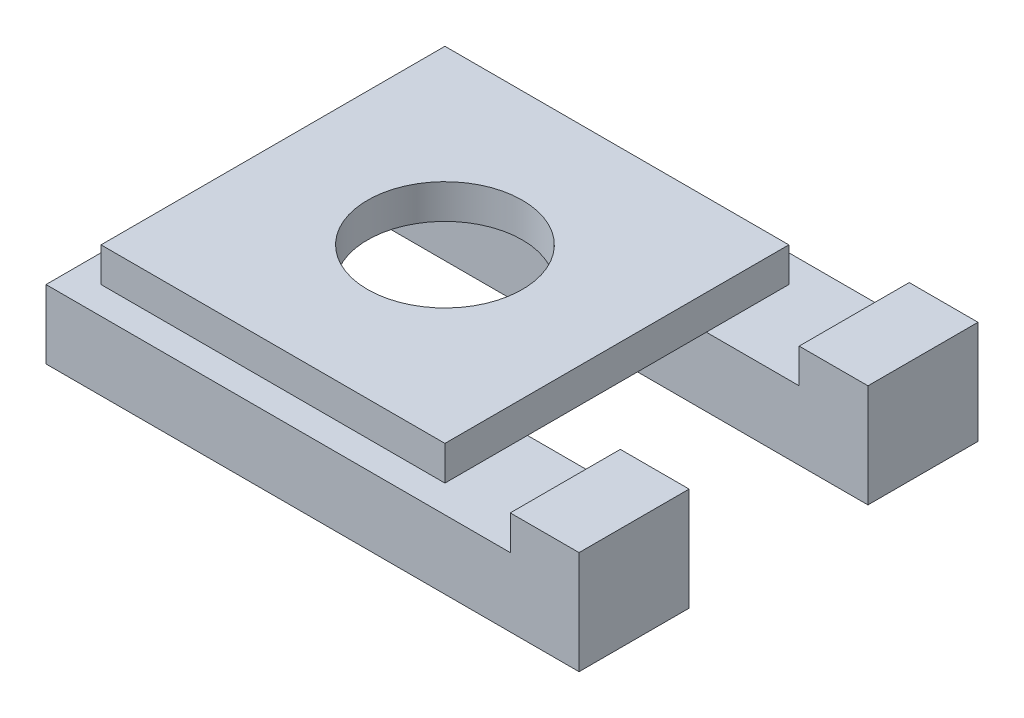
ISO-10303-21;
HEADER;
FILE_DESCRIPTION(('STEP AP214'),'2;1');
FILE_NAME('part.step','',(''),(''),'','','');
FILE_SCHEMA(('AUTOMOTIVE_DESIGN { 1 0 10303 214 1 1 1 1 }'));
ENDSEC;
DATA;
#1=APPLICATION_CONTEXT('core data for automotive mechanical design processes');
#2=APPLICATION_PROTOCOL_DEFINITION('international standard','automotive_design',2000,#1);
#3=PRODUCT_CONTEXT('',#1,'mechanical');
#4=PRODUCT('Part','Part','',(#3));
#5=PRODUCT_RELATED_PRODUCT_CATEGORY('part','',(#4));
#6=PRODUCT_DEFINITION_FORMATION('','',#4);
#7=PRODUCT_DEFINITION_CONTEXT('part definition',#1,'design');
#8=PRODUCT_DEFINITION('design','',#6,#7);
#9=PRODUCT_DEFINITION_SHAPE('','',#8);
#10=(LENGTH_UNIT() NAMED_UNIT(*) SI_UNIT(.MILLI.,.METRE.));
#11=(NAMED_UNIT(*) PLANE_ANGLE_UNIT() SI_UNIT($,.RADIAN.));
#12=(NAMED_UNIT(*) SI_UNIT($,.STERADIAN.) SOLID_ANGLE_UNIT());
#13=UNCERTAINTY_MEASURE_WITH_UNIT(LENGTH_MEASURE(1.E-05),#10,'distance_accuracy_value','');
#14=(GEOMETRIC_REPRESENTATION_CONTEXT(3) GLOBAL_UNCERTAINTY_ASSIGNED_CONTEXT((#13)) GLOBAL_UNIT_ASSIGNED_CONTEXT((#10,
#11,#12)) REPRESENTATION_CONTEXT('',''));
#15=CARTESIAN_POINT('',(0.,0.,0.));
#16=DIRECTION('',(0.,0.,1.));
#17=DIRECTION('',(1.,0.,0.));
#18=AXIS2_PLACEMENT_3D('',#15,#16,#17);
#19=CARTESIAN_POINT('',(0.,0.,0.));
#20=DIRECTION('',(0.,-1.,0.));
#21=DIRECTION('',(0.,0.,-1.));
#22=AXIS2_PLACEMENT_3D('',#19,#20,#21);
#23=PLANE('',#22);
#24=DIRECTION('',(0.,0.,1.));
#25=VECTOR('',#24,1.);
#26=CARTESIAN_POINT('',(77.,0.,-58.));
#27=LINE('',#26,#25);
#28=CARTESIAN_POINT('',(77.,0.,-58.));
#29=VERTEX_POINT('',#28);
#30=CARTESIAN_POINT('',(77.,0.,-26.));
#31=VERTEX_POINT('',#30);
#32=EDGE_CURVE('E192',#29,#31,#27,.T.);
#33=ORIENTED_EDGE('',*,*,#32,.F.);
#34=DIRECTION('',(1.,0.,0.));
#35=VECTOR('',#34,1.);
#36=CARTESIAN_POINT('',(-58.,0.,-58.));
#37=LINE('',#36,#35);
#38=CARTESIAN_POINT('',(-58.,0.,-58.));
#39=VERTEX_POINT('',#38);
#40=EDGE_CURVE('E204',#39,#29,#37,.T.);
#41=ORIENTED_EDGE('',*,*,#40,.F.);
#42=DIRECTION('',(0.,0.,-1.));
#43=VECTOR('',#42,1.);
#44=CARTESIAN_POINT('',(-58.,0.,-58.));
#45=LINE('',#44,#43);
#46=CARTESIAN_POINT('',(-58.,0.,-26.));
#47=VERTEX_POINT('',#46);
#48=EDGE_CURVE('E248',#47,#39,#45,.T.);
#49=ORIENTED_EDGE('',*,*,#48,.F.);
#50=DIRECTION('',(-1.,0.,0.));
#51=VECTOR('',#50,1.);
#52=CARTESIAN_POINT('',(-58.,0.,-26.));
#53=LINE('',#52,#51);
#54=CARTESIAN_POINT('',(-50.,0.,-26.));
#55=VERTEX_POINT('',#54);
#56=EDGE_CURVE('E255',#55,#47,#53,.T.);
#57=ORIENTED_EDGE('',*,*,#56,.F.);
#58=DIRECTION('',(0.,0.,1.));
#59=VECTOR('',#58,1.);
#60=CARTESIAN_POINT('',(-50.,0.,50.));
#61=LINE('',#60,#59);
#62=CARTESIAN_POINT('',(-50.,0.,-50.));
#63=VERTEX_POINT('',#62);
#64=EDGE_CURVE('E290',#63,#55,#61,.T.);
#65=ORIENTED_EDGE('',*,*,#64,.F.);
#66=DIRECTION('',(-1.,0.,0.));
#67=VECTOR('',#66,1.);
#68=CARTESIAN_POINT('',(-50.,0.,-50.));
#69=LINE('',#68,#67);
#70=CARTESIAN_POINT('',(50.,0.,-50.));
#71=VERTEX_POINT('',#70);
#72=EDGE_CURVE('E284',#71,#63,#69,.T.);
#73=ORIENTED_EDGE('',*,*,#72,.F.);
#74=DIRECTION('',(0.,0.,-1.));
#75=VECTOR('',#74,1.);
#76=CARTESIAN_POINT('',(50.,0.,50.));
#77=LINE('',#76,#75);
#78=CARTESIAN_POINT('',(50.,0.,-26.));
#79=VERTEX_POINT('',#78);
#80=EDGE_CURVE('E270',#79,#71,#77,.T.);
#81=ORIENTED_EDGE('',*,*,#80,.F.);
#82=EDGE_CURVE('E254',#31,#79,#53,.T.);
#83=ORIENTED_EDGE('',*,*,#82,.F.);
#84=EDGE_LOOP('',(#33,#41,#49,#57,#65,#73,#81,#83));
#85=FACE_BOUND('',#84,.T.);
#86=ADVANCED_FACE('F39',(#85),#23,.F.);
#87=CARTESIAN_POINT('',(0.,0.,0.));
#88=DIRECTION('',(0.,-1.,0.));
#89=DIRECTION('',(0.,0.,-1.));
#90=AXIS2_PLACEMENT_3D('',#87,#88,#89);
#91=PLANE('',#90);
#92=DIRECTION('',(0.,0.,1.));
#93=VECTOR('',#92,1.);
#94=CARTESIAN_POINT('',(77.,0.,26.));
#95=LINE('',#94,#93);
#96=CARTESIAN_POINT('',(77.,0.,26.));
#97=VERTEX_POINT('',#96);
#98=CARTESIAN_POINT('',(77.,0.,58.));
#99=VERTEX_POINT('',#98);
#100=EDGE_CURVE('E197',#97,#99,#95,.T.);
#101=ORIENTED_EDGE('',*,*,#100,.F.);
#102=DIRECTION('',(1.,0.,0.));
#103=VECTOR('',#102,1.);
#104=CARTESIAN_POINT('',(-58.,0.,26.));
#105=LINE('',#104,#103);
#106=CARTESIAN_POINT('',(50.,0.,26.));
#107=VERTEX_POINT('',#106);
#108=EDGE_CURVE('E51',#107,#97,#105,.T.);
#109=ORIENTED_EDGE('',*,*,#108,.F.);
#110=CARTESIAN_POINT('',(50.,0.,50.));
#111=VERTEX_POINT('',#110);
#112=EDGE_CURVE('E281',#111,#107,#77,.T.);
#113=ORIENTED_EDGE('',*,*,#112,.F.);
#114=DIRECTION('',(1.,0.,0.));
#115=VECTOR('',#114,1.);
#116=CARTESIAN_POINT('',(-50.,0.,50.));
#117=LINE('',#116,#115);
#118=CARTESIAN_POINT('',(-50.,0.,50.));
#119=VERTEX_POINT('',#118);
#120=EDGE_CURVE('E273',#119,#111,#117,.T.);
#121=ORIENTED_EDGE('',*,*,#120,.F.);
#122=CARTESIAN_POINT('',(-50.,0.,26.));
#123=VERTEX_POINT('',#122);
#124=EDGE_CURVE('E288',#123,#119,#61,.T.);
#125=ORIENTED_EDGE('',*,*,#124,.F.);
#126=CARTESIAN_POINT('',(-58.,0.,26.));
#127=VERTEX_POINT('',#126);
#128=EDGE_CURVE('E49',#127,#123,#105,.T.);
#129=ORIENTED_EDGE('',*,*,#128,.F.);
#130=DIRECTION('',(0.,0.,-1.));
#131=VECTOR('',#130,1.);
#132=CARTESIAN_POINT('',(-58.,0.,58.));
#133=LINE('',#132,#131);
#134=CARTESIAN_POINT('',(-58.,0.,58.));
#135=VERTEX_POINT('',#134);
#136=EDGE_CURVE('E177',#135,#127,#133,.T.);
#137=ORIENTED_EDGE('',*,*,#136,.F.);
#138=DIRECTION('',(-1.,0.,0.));
#139=VECTOR('',#138,1.);
#140=CARTESIAN_POINT('',(-58.,0.,58.));
#141=LINE('',#140,#139);
#142=EDGE_CURVE('E224',#99,#135,#141,.T.);
#143=ORIENTED_EDGE('',*,*,#142,.F.);
#144=EDGE_LOOP('',(#101,#109,#113,#121,#125,#129,#137,#143));
#145=FACE_BOUND('',#144,.T.);
#146=ADVANCED_FACE('F333',(#145),#91,.F.);
#147=CARTESIAN_POINT('',(0.,10.,0.));
#148=DIRECTION('',(0.,-1.,0.));
#149=DIRECTION('',(0.,0.,-1.));
#150=AXIS2_PLACEMENT_3D('',#147,#148,#149);
#151=PLANE('',#150);
#152=DIRECTION('',(0.,0.,-1.));
#153=VECTOR('',#152,1.);
#154=CARTESIAN_POINT('',(50.,10.,50.));
#155=LINE('',#154,#153);
#156=CARTESIAN_POINT('',(50.,10.,50.));
#157=VERTEX_POINT('',#156);
#158=CARTESIAN_POINT('',(50.,10.,-50.));
#159=VERTEX_POINT('',#158);
#160=EDGE_CURVE('E269',#157,#159,#155,.T.);
#161=ORIENTED_EDGE('',*,*,#160,.T.);
#162=DIRECTION('',(-1.,0.,0.));
#163=VECTOR('',#162,1.);
#164=CARTESIAN_POINT('',(-50.,10.,-50.));
#165=LINE('',#164,#163);
#166=CARTESIAN_POINT('',(-50.,10.,-50.));
#167=VERTEX_POINT('',#166);
#168=EDGE_CURVE('E272',#159,#167,#165,.T.);
#169=ORIENTED_EDGE('',*,*,#168,.T.);
#170=DIRECTION('',(0.,0.,1.));
#171=VECTOR('',#170,1.);
#172=CARTESIAN_POINT('',(-50.,10.,50.));
#173=LINE('',#172,#171);
#174=CARTESIAN_POINT('',(-50.,10.,50.));
#175=VERTEX_POINT('',#174);
#176=EDGE_CURVE('E277',#167,#175,#173,.T.);
#177=ORIENTED_EDGE('',*,*,#176,.T.);
#178=DIRECTION('',(1.,0.,0.));
#179=VECTOR('',#178,1.);
#180=CARTESIAN_POINT('',(-50.,10.,50.));
#181=LINE('',#180,#179);
#182=EDGE_CURVE('E279',#175,#157,#181,.T.);
#183=ORIENTED_EDGE('',*,*,#182,.T.);
#184=EDGE_LOOP('',(#161,#169,#177,#183));
#185=FACE_BOUND('',#184,.T.);
#186=CARTESIAN_POINT('',(0.,10.,0.));
#187=DIRECTION('',(0.,1.,0.));
#188=DIRECTION('',(0.,0.,1.));
#189=AXIS2_PLACEMENT_3D('',#186,#187,#188);
#190=CIRCLE('',#189,22.5);
#191=CARTESIAN_POINT('',(0.,10.,22.5));
#192=VERTEX_POINT('',#191);
#193=EDGE_CURVE('E262',#192,#192,#190,.T.);
#194=ORIENTED_EDGE('',*,*,#193,.F.);
#195=EDGE_LOOP('',(#194));
#196=FACE_BOUND('',#195,.T.);
#197=ADVANCED_FACE('F340',(#185,#196),#151,.F.);
#198=CARTESIAN_POINT('',(0.,0.,0.));
#199=DIRECTION('',(0.,-1.,0.));
#200=DIRECTION('',(0.,0.,-1.));
#201=AXIS2_PLACEMENT_3D('',#198,#199,#200);
#202=PLANE('',#201);
#203=EDGE_CURVE('E11',#123,#107,#105,.T.);
#204=ORIENTED_EDGE('',*,*,#203,.F.);
#205=EDGE_CURVE('E289',#55,#123,#61,.T.);
#206=ORIENTED_EDGE('',*,*,#205,.F.);
#207=EDGE_CURVE('E48',#79,#55,#53,.T.);
#208=ORIENTED_EDGE('',*,*,#207,.F.);
#209=EDGE_CURVE('E283',#107,#79,#77,.T.);
#210=ORIENTED_EDGE('',*,*,#209,.F.);
#211=EDGE_LOOP('',(#204,#206,#208,#210));
#212=FACE_BOUND('',#211,.T.);
#213=CARTESIAN_POINT('',(0.,0.,0.));
#214=DIRECTION('',(0.,1.,0.));
#215=DIRECTION('',(0.,0.,1.));
#216=AXIS2_PLACEMENT_3D('',#213,#214,#215);
#217=CIRCLE('',#216,22.5);
#218=CARTESIAN_POINT('',(0.,0.,22.5));
#219=VERTEX_POINT('',#218);
#220=EDGE_CURVE('E244',#219,#219,#217,.T.);
#221=ORIENTED_EDGE('',*,*,#220,.T.);
#222=EDGE_LOOP('',(#221));
#223=FACE_BOUND('',#222,.T.);
#224=ADVANCED_FACE('F360',(#212,#223),#202,.T.);
#225=CARTESIAN_POINT('',(50.,10.,50.));
#226=DIRECTION('',(-1.,0.,0.));
#227=DIRECTION('',(0.,0.,1.));
#228=AXIS2_PLACEMENT_3D('',#225,#226,#227);
#229=PLANE('',#228);
#230=ORIENTED_EDGE('',*,*,#112,.T.);
#231=ORIENTED_EDGE('',*,*,#209,.T.);
#232=ORIENTED_EDGE('',*,*,#80,.T.);
#233=DIRECTION('',(0.,-1.,0.));
#234=VECTOR('',#233,1.);
#235=CARTESIAN_POINT('',(50.,10.,-50.));
#236=LINE('',#235,#234);
#237=EDGE_CURVE('E43',#159,#71,#236,.T.);
#238=ORIENTED_EDGE('',*,*,#237,.F.);
#239=ORIENTED_EDGE('',*,*,#160,.F.);
#240=DIRECTION('',(0.,-1.,0.));
#241=VECTOR('',#240,1.);
#242=CARTESIAN_POINT('',(50.,10.,50.));
#243=LINE('',#242,#241);
#244=EDGE_CURVE('E278',#157,#111,#243,.T.);
#245=ORIENTED_EDGE('',*,*,#244,.T.);
#246=EDGE_LOOP('',(#230,#231,#232,#238,#239,#245));
#247=FACE_BOUND('',#246,.T.);
#248=ADVANCED_FACE('F41',(#247),#229,.F.);
#249=CARTESIAN_POINT('',(-50.,10.,-50.));
#250=DIRECTION('',(0.,0.,1.));
#251=DIRECTION('',(1.,0.,0.));
#252=AXIS2_PLACEMENT_3D('',#249,#250,#251);
#253=PLANE('',#252);
#254=ORIENTED_EDGE('',*,*,#72,.T.);
#255=DIRECTION('',(0.,-1.,0.));
#256=VECTOR('',#255,1.);
#257=CARTESIAN_POINT('',(-50.,10.,-50.));
#258=LINE('',#257,#256);
#259=EDGE_CURVE('E293',#167,#63,#258,.T.);
#260=ORIENTED_EDGE('',*,*,#259,.F.);
#261=ORIENTED_EDGE('',*,*,#168,.F.);
#262=ORIENTED_EDGE('',*,*,#237,.T.);
#263=EDGE_LOOP('',(#254,#260,#261,#262));
#264=FACE_BOUND('',#263,.T.);
#265=ADVANCED_FACE('F370',(#264),#253,.F.);
#266=CARTESIAN_POINT('',(-50.,10.,50.));
#267=DIRECTION('',(1.,0.,0.));
#268=DIRECTION('',(0.,0.,-1.));
#269=AXIS2_PLACEMENT_3D('',#266,#267,#268);
#270=PLANE('',#269);
#271=ORIENTED_EDGE('',*,*,#64,.T.);
#272=ORIENTED_EDGE('',*,*,#205,.T.);
#273=ORIENTED_EDGE('',*,*,#124,.T.);
#274=DIRECTION('',(0.,-1.,0.));
#275=VECTOR('',#274,1.);
#276=CARTESIAN_POINT('',(-50.,10.,50.));
#277=LINE('',#276,#275);
#278=EDGE_CURVE('E291',#175,#119,#277,.T.);
#279=ORIENTED_EDGE('',*,*,#278,.F.);
#280=ORIENTED_EDGE('',*,*,#176,.F.);
#281=ORIENTED_EDGE('',*,*,#259,.T.);
#282=EDGE_LOOP('',(#271,#272,#273,#279,#280,#281));
#283=FACE_BOUND('',#282,.T.);
#284=ADVANCED_FACE('F365',(#283),#270,.F.);
#285=CARTESIAN_POINT('',(-50.,10.,50.));
#286=DIRECTION('',(0.,0.,-1.));
#287=DIRECTION('',(-1.,0.,0.));
#288=AXIS2_PLACEMENT_3D('',#285,#286,#287);
#289=PLANE('',#288);
#290=ORIENTED_EDGE('',*,*,#120,.T.);
#291=ORIENTED_EDGE('',*,*,#244,.F.);
#292=ORIENTED_EDGE('',*,*,#182,.F.);
#293=ORIENTED_EDGE('',*,*,#278,.T.);
#294=EDGE_LOOP('',(#290,#291,#292,#293));
#295=FACE_BOUND('',#294,.T.);
#296=ADVANCED_FACE('F354',(#295),#289,.F.);
#297=CARTESIAN_POINT('',(0.,10.,0.));
#298=DIRECTION('',(0.,-1.,0.));
#299=DIRECTION('',(0.,0.,-1.));
#300=AXIS2_PLACEMENT_3D('',#297,#298,#299);
#301=CYLINDRICAL_SURFACE('',#300,22.5);
#302=ORIENTED_EDGE('',*,*,#193,.T.);
#303=EDGE_LOOP('',(#302));
#304=FACE_BOUND('',#303,.T.);
#305=ORIENTED_EDGE('',*,*,#220,.F.);
#306=EDGE_LOOP('',(#305));
#307=FACE_BOUND('',#306,.T.);
#308=ADVANCED_FACE('F348',(#304,#307),#301,.F.);
#309=CARTESIAN_POINT('',(-58.,-20.,-58.));
#310=DIRECTION('',(0.,0.,1.));
#311=DIRECTION('',(1.,0.,0.));
#312=AXIS2_PLACEMENT_3D('',#309,#310,#311);
#313=PLANE('',#312);
#314=ORIENTED_EDGE('',*,*,#40,.T.);
#315=DIRECTION('',(0.,-1.,0.));
#316=VECTOR('',#315,1.);
#317=CARTESIAN_POINT('',(77.,10.,-58.));
#318=LINE('',#317,#316);
#319=CARTESIAN_POINT('',(77.,10.,-58.));
#320=VERTEX_POINT('',#319);
#321=EDGE_CURVE('E187',#320,#29,#318,.T.);
#322=ORIENTED_EDGE('',*,*,#321,.F.);
#323=DIRECTION('',(-1.,0.,0.));
#324=VECTOR('',#323,1.);
#325=CARTESIAN_POINT('',(97.,10.,-58.));
#326=LINE('',#325,#324);
#327=CARTESIAN_POINT('',(97.,10.,-58.));
#328=VERTEX_POINT('',#327);
#329=EDGE_CURVE('E184',#328,#320,#326,.T.);
#330=ORIENTED_EDGE('',*,*,#329,.F.);
#331=DIRECTION('',(0.,1.,0.));
#332=VECTOR('',#331,1.);
#333=CARTESIAN_POINT('',(97.,-20.,-58.));
#334=LINE('',#333,#332);
#335=CARTESIAN_POINT('',(97.,-20.,-58.));
#336=VERTEX_POINT('',#335);
#337=EDGE_CURVE('E168',#336,#328,#334,.T.);
#338=ORIENTED_EDGE('',*,*,#337,.F.);
#339=DIRECTION('',(1.,0.,0.));
#340=VECTOR('',#339,1.);
#341=CARTESIAN_POINT('',(-58.,-20.,-58.));
#342=LINE('',#341,#340);
#343=CARTESIAN_POINT('',(-58.,-20.,-58.));
#344=VERTEX_POINT('',#343);
#345=EDGE_CURVE('E243',#344,#336,#342,.T.);
#346=ORIENTED_EDGE('',*,*,#345,.F.);
#347=DIRECTION('',(0.,1.,0.));
#348=VECTOR('',#347,1.);
#349=CARTESIAN_POINT('',(-58.,-20.,-58.));
#350=LINE('',#349,#348);
#351=EDGE_CURVE('E252',#344,#39,#350,.T.);
#352=ORIENTED_EDGE('',*,*,#351,.T.);
#353=EDGE_LOOP('',(#314,#322,#330,#338,#346,#352));
#354=FACE_BOUND('',#353,.T.);
#355=ADVANCED_FACE('F186',(#354),#313,.F.);
#356=CARTESIAN_POINT('',(97.,-20.,-58.));
#357=DIRECTION('',(-1.,0.,0.));
#358=DIRECTION('',(0.,0.,1.));
#359=AXIS2_PLACEMENT_3D('',#356,#357,#358);
#360=PLANE('',#359);
#361=ORIENTED_EDGE('',*,*,#337,.T.);
#362=DIRECTION('',(0.,0.,-1.));
#363=VECTOR('',#362,1.);
#364=CARTESIAN_POINT('',(97.,10.,-58.));
#365=LINE('',#364,#363);
#366=CARTESIAN_POINT('',(97.,10.,-26.));
#367=VERTEX_POINT('',#366);
#368=EDGE_CURVE('E175',#367,#328,#365,.T.);
#369=ORIENTED_EDGE('',*,*,#368,.F.);
#370=DIRECTION('',(0.,1.,0.));
#371=VECTOR('',#370,1.);
#372=CARTESIAN_POINT('',(97.,-20.,-26.));
#373=LINE('',#372,#371);
#374=CARTESIAN_POINT('',(97.,-20.,-26.));
#375=VERTEX_POINT('',#374);
#376=EDGE_CURVE('E182',#375,#367,#373,.T.);
#377=ORIENTED_EDGE('',*,*,#376,.F.);
#378=DIRECTION('',(0.,0.,1.));
#379=VECTOR('',#378,1.);
#380=CARTESIAN_POINT('',(97.,-20.,-58.));
#381=LINE('',#380,#379);
#382=EDGE_CURVE('E178',#336,#375,#381,.T.);
#383=ORIENTED_EDGE('',*,*,#382,.F.);
#384=EDGE_LOOP('',(#361,#369,#377,#383));
#385=FACE_BOUND('',#384,.T.);
#386=ADVANCED_FACE('F172',(#385),#360,.F.);
#387=CARTESIAN_POINT('',(-58.,-20.,-26.));
#388=DIRECTION('',(0.,0.,-1.));
#389=DIRECTION('',(-1.,0.,0.));
#390=AXIS2_PLACEMENT_3D('',#387,#388,#389);
#391=PLANE('',#390);
#392=ORIENTED_EDGE('',*,*,#376,.T.);
#393=DIRECTION('',(1.,0.,0.));
#394=VECTOR('',#393,1.);
#395=CARTESIAN_POINT('',(97.,10.,-26.));
#396=LINE('',#395,#394);
#397=CARTESIAN_POINT('',(77.,10.,-26.));
#398=VERTEX_POINT('',#397);
#399=EDGE_CURVE('E194',#398,#367,#396,.T.);
#400=ORIENTED_EDGE('',*,*,#399,.F.);
#401=DIRECTION('',(0.,-1.,0.));
#402=VECTOR('',#401,1.);
#403=CARTESIAN_POINT('',(77.,10.,-26.));
#404=LINE('',#403,#402);
#405=EDGE_CURVE('E59',#398,#31,#404,.T.);
#406=ORIENTED_EDGE('',*,*,#405,.T.);
#407=ORIENTED_EDGE('',*,*,#82,.T.);
#408=ORIENTED_EDGE('',*,*,#207,.T.);
#409=ORIENTED_EDGE('',*,*,#56,.T.);
#410=DIRECTION('',(0.,1.,0.));
#411=VECTOR('',#410,1.);
#412=CARTESIAN_POINT('',(-58.,-20.,-26.));
#413=LINE('',#412,#411);
#414=CARTESIAN_POINT('',(-58.,-20.,-26.));
#415=VERTEX_POINT('',#414);
#416=EDGE_CURVE('E257',#415,#47,#413,.T.);
#417=ORIENTED_EDGE('',*,*,#416,.F.);
#418=DIRECTION('',(-1.,0.,0.));
#419=VECTOR('',#418,1.);
#420=CARTESIAN_POINT('',(-58.,-20.,-26.));
#421=LINE('',#420,#419);
#422=EDGE_CURVE('E246',#375,#415,#421,.T.);
#423=ORIENTED_EDGE('',*,*,#422,.F.);
#424=EDGE_LOOP('',(#392,#400,#406,#407,#408,#409,#417,#423));
#425=FACE_BOUND('',#424,.T.);
#426=ADVANCED_FACE('F310',(#425),#391,.F.);
#427=CARTESIAN_POINT('',(-58.,-20.,-58.));
#428=DIRECTION('',(1.,0.,0.));
#429=DIRECTION('',(0.,0.,-1.));
#430=AXIS2_PLACEMENT_3D('',#427,#428,#429);
#431=PLANE('',#430);
#432=ORIENTED_EDGE('',*,*,#48,.T.);
#433=ORIENTED_EDGE('',*,*,#351,.F.);
#434=DIRECTION('',(0.,0.,-1.));
#435=VECTOR('',#434,1.);
#436=CARTESIAN_POINT('',(-58.,-20.,-58.));
#437=LINE('',#436,#435);
#438=EDGE_CURVE('E247',#415,#344,#437,.T.);
#439=ORIENTED_EDGE('',*,*,#438,.F.);
#440=ORIENTED_EDGE('',*,*,#416,.T.);
#441=EDGE_LOOP('',(#432,#433,#439,#440));
#442=FACE_BOUND('',#441,.T.);
#443=ADVANCED_FACE('F312',(#442),#431,.F.);
#444=CARTESIAN_POINT('',(0.,-20.,0.));
#445=DIRECTION('',(0.,-1.,0.));
#446=DIRECTION('',(0.,0.,-1.));
#447=AXIS2_PLACEMENT_3D('',#444,#445,#446);
#448=PLANE('',#447);
#449=ORIENTED_EDGE('',*,*,#345,.T.);
#450=ORIENTED_EDGE('',*,*,#382,.T.);
#451=ORIENTED_EDGE('',*,*,#422,.T.);
#452=ORIENTED_EDGE('',*,*,#438,.T.);
#453=EDGE_LOOP('',(#449,#450,#451,#452));
#454=FACE_BOUND('',#453,.T.);
#455=ADVANCED_FACE('F321',(#454),#448,.T.);
#456=CARTESIAN_POINT('',(-58.,-20.,58.));
#457=DIRECTION('',(1.,0.,0.));
#458=DIRECTION('',(0.,0.,-1.));
#459=AXIS2_PLACEMENT_3D('',#456,#457,#458);
#460=PLANE('',#459);
#461=ORIENTED_EDGE('',*,*,#136,.T.);
#462=DIRECTION('',(0.,1.,0.));
#463=VECTOR('',#462,1.);
#464=CARTESIAN_POINT('',(-58.,-20.,26.));
#465=LINE('',#464,#463);
#466=CARTESIAN_POINT('',(-58.,-20.,26.));
#467=VERTEX_POINT('',#466);
#468=EDGE_CURVE('E238',#467,#127,#465,.T.);
#469=ORIENTED_EDGE('',*,*,#468,.F.);
#470=DIRECTION('',(0.,0.,-1.));
#471=VECTOR('',#470,1.);
#472=CARTESIAN_POINT('',(-58.,-20.,58.));
#473=LINE('',#472,#471);
#474=CARTESIAN_POINT('',(-58.,-20.,58.));
#475=VERTEX_POINT('',#474);
#476=EDGE_CURVE('E218',#475,#467,#473,.T.);
#477=ORIENTED_EDGE('',*,*,#476,.F.);
#478=DIRECTION('',(0.,1.,0.));
#479=VECTOR('',#478,1.);
#480=CARTESIAN_POINT('',(-58.,-20.,58.));
#481=LINE('',#480,#479);
#482=EDGE_CURVE('E228',#475,#135,#481,.T.);
#483=ORIENTED_EDGE('',*,*,#482,.T.);
#484=EDGE_LOOP('',(#461,#469,#477,#483));
#485=FACE_BOUND('',#484,.T.);
#486=ADVANCED_FACE('F323',(#485),#460,.F.);
#487=CARTESIAN_POINT('',(-58.,-20.,26.));
#488=DIRECTION('',(0.,0.,1.));
#489=DIRECTION('',(1.,0.,0.));
#490=AXIS2_PLACEMENT_3D('',#487,#488,#489);
#491=PLANE('',#490);
#492=ORIENTED_EDGE('',*,*,#128,.T.);
#493=ORIENTED_EDGE('',*,*,#203,.T.);
#494=ORIENTED_EDGE('',*,*,#108,.T.);
#495=DIRECTION('',(0.,-1.,0.));
#496=VECTOR('',#495,1.);
#497=CARTESIAN_POINT('',(77.,10.,26.));
#498=LINE('',#497,#496);
#499=CARTESIAN_POINT('',(77.,10.,26.));
#500=VERTEX_POINT('',#499);
#501=EDGE_CURVE('E202',#500,#97,#498,.T.);
#502=ORIENTED_EDGE('',*,*,#501,.F.);
#503=DIRECTION('',(-1.,0.,0.));
#504=VECTOR('',#503,1.);
#505=CARTESIAN_POINT('',(97.,10.,26.));
#506=LINE('',#505,#504);
#507=CARTESIAN_POINT('',(97.,10.,26.));
#508=VERTEX_POINT('',#507);
#509=EDGE_CURVE('E214',#508,#500,#506,.T.);
#510=ORIENTED_EDGE('',*,*,#509,.F.);
#511=DIRECTION('',(0.,1.,0.));
#512=VECTOR('',#511,1.);
#513=CARTESIAN_POINT('',(97.,-20.,26.));
#514=LINE('',#513,#512);
#515=CARTESIAN_POINT('',(97.,-20.,26.));
#516=VERTEX_POINT('',#515);
#517=EDGE_CURVE('E236',#516,#508,#514,.T.);
#518=ORIENTED_EDGE('',*,*,#517,.F.);
#519=DIRECTION('',(1.,0.,0.));
#520=VECTOR('',#519,1.);
#521=CARTESIAN_POINT('',(-58.,-20.,26.));
#522=LINE('',#521,#520);
#523=EDGE_CURVE('E225',#467,#516,#522,.T.);
#524=ORIENTED_EDGE('',*,*,#523,.F.);
#525=ORIENTED_EDGE('',*,*,#468,.T.);
#526=EDGE_LOOP('',(#492,#493,#494,#502,#510,#518,#524,#525));
#527=FACE_BOUND('',#526,.T.);
#528=ADVANCED_FACE('F328',(#527),#491,.F.);
#529=CARTESIAN_POINT('',(97.,-20.,58.));
#530=DIRECTION('',(-1.,0.,0.));
#531=DIRECTION('',(0.,0.,1.));
#532=AXIS2_PLACEMENT_3D('',#529,#530,#531);
#533=PLANE('',#532);
#534=ORIENTED_EDGE('',*,*,#517,.T.);
#535=DIRECTION('',(0.,0.,-1.));
#536=VECTOR('',#535,1.);
#537=CARTESIAN_POINT('',(97.,10.,26.));
#538=LINE('',#537,#536);
#539=CARTESIAN_POINT('',(97.,10.,58.));
#540=VERTEX_POINT('',#539);
#541=EDGE_CURVE('E209',#540,#508,#538,.T.);
#542=ORIENTED_EDGE('',*,*,#541,.F.);
#543=DIRECTION('',(0.,1.,0.));
#544=VECTOR('',#543,1.);
#545=CARTESIAN_POINT('',(97.,-20.,58.));
#546=LINE('',#545,#544);
#547=CARTESIAN_POINT('',(97.,-20.,58.));
#548=VERTEX_POINT('',#547);
#549=EDGE_CURVE('E237',#548,#540,#546,.T.);
#550=ORIENTED_EDGE('',*,*,#549,.F.);
#551=DIRECTION('',(0.,0.,1.));
#552=VECTOR('',#551,1.);
#553=CARTESIAN_POINT('',(97.,-20.,58.));
#554=LINE('',#553,#552);
#555=EDGE_CURVE('E223',#516,#548,#554,.T.);
#556=ORIENTED_EDGE('',*,*,#555,.F.);
#557=EDGE_LOOP('',(#534,#542,#550,#556));
#558=FACE_BOUND('',#557,.T.);
#559=ADVANCED_FACE('F408',(#558),#533,.F.);
#560=CARTESIAN_POINT('',(-58.,-20.,58.));
#561=DIRECTION('',(0.,0.,-1.));
#562=DIRECTION('',(-1.,0.,0.));
#563=AXIS2_PLACEMENT_3D('',#560,#561,#562);
#564=PLANE('',#563);
#565=ORIENTED_EDGE('',*,*,#549,.T.);
#566=DIRECTION('',(1.,0.,0.));
#567=VECTOR('',#566,1.);
#568=CARTESIAN_POINT('',(97.,10.,58.));
#569=LINE('',#568,#567);
#570=CARTESIAN_POINT('',(77.,10.,58.));
#571=VERTEX_POINT('',#570);
#572=EDGE_CURVE('E208',#571,#540,#569,.T.);
#573=ORIENTED_EDGE('',*,*,#572,.F.);
#574=DIRECTION('',(0.,-1.,0.));
#575=VECTOR('',#574,1.);
#576=CARTESIAN_POINT('',(77.,10.,58.));
#577=LINE('',#576,#575);
#578=EDGE_CURVE('E68',#571,#99,#577,.T.);
#579=ORIENTED_EDGE('',*,*,#578,.T.);
#580=ORIENTED_EDGE('',*,*,#142,.T.);
#581=ORIENTED_EDGE('',*,*,#482,.F.);
#582=DIRECTION('',(-1.,0.,0.));
#583=VECTOR('',#582,1.);
#584=CARTESIAN_POINT('',(-58.,-20.,58.));
#585=LINE('',#584,#583);
#586=EDGE_CURVE('E227',#548,#475,#585,.T.);
#587=ORIENTED_EDGE('',*,*,#586,.F.);
#588=EDGE_LOOP('',(#565,#573,#579,#580,#581,#587));
#589=FACE_BOUND('',#588,.T.);
#590=ADVANCED_FACE('F402',(#589),#564,.F.);
#591=CARTESIAN_POINT('',(0.,-20.,0.));
#592=DIRECTION('',(0.,-1.,0.));
#593=DIRECTION('',(0.,0.,-1.));
#594=AXIS2_PLACEMENT_3D('',#591,#592,#593);
#595=PLANE('',#594);
#596=ORIENTED_EDGE('',*,*,#476,.T.);
#597=ORIENTED_EDGE('',*,*,#523,.T.);
#598=ORIENTED_EDGE('',*,*,#555,.T.);
#599=ORIENTED_EDGE('',*,*,#586,.T.);
#600=EDGE_LOOP('',(#596,#597,#598,#599));
#601=FACE_BOUND('',#600,.T.);
#602=ADVANCED_FACE('F404',(#601),#595,.T.);
#603=CARTESIAN_POINT('',(77.,10.,26.));
#604=DIRECTION('',(1.,0.,0.));
#605=DIRECTION('',(0.,0.,-1.));
#606=AXIS2_PLACEMENT_3D('',#603,#604,#605);
#607=PLANE('',#606);
#608=ORIENTED_EDGE('',*,*,#100,.T.);
#609=ORIENTED_EDGE('',*,*,#578,.F.);
#610=DIRECTION('',(0.,0.,1.));
#611=VECTOR('',#610,1.);
#612=CARTESIAN_POINT('',(77.,10.,26.));
#613=LINE('',#612,#611);
#614=EDGE_CURVE('E213',#500,#571,#613,.T.);
#615=ORIENTED_EDGE('',*,*,#614,.F.);
#616=ORIENTED_EDGE('',*,*,#501,.T.);
#617=EDGE_LOOP('',(#608,#609,#615,#616));
#618=FACE_BOUND('',#617,.T.);
#619=ADVANCED_FACE('F412',(#618),#607,.F.);
#620=CARTESIAN_POINT('',(0.,10.,0.));
#621=DIRECTION('',(0.,-1.,0.));
#622=DIRECTION('',(0.,0.,-1.));
#623=AXIS2_PLACEMENT_3D('',#620,#621,#622);
#624=PLANE('',#623);
#625=ORIENTED_EDGE('',*,*,#541,.T.);
#626=ORIENTED_EDGE('',*,*,#509,.T.);
#627=ORIENTED_EDGE('',*,*,#614,.T.);
#628=ORIENTED_EDGE('',*,*,#572,.T.);
#629=EDGE_LOOP('',(#625,#626,#627,#628));
#630=FACE_BOUND('',#629,.T.);
#631=ADVANCED_FACE('F415',(#630),#624,.F.);
#632=CARTESIAN_POINT('',(77.,10.,-58.));
#633=DIRECTION('',(1.,0.,0.));
#634=DIRECTION('',(0.,0.,-1.));
#635=AXIS2_PLACEMENT_3D('',#632,#633,#634);
#636=PLANE('',#635);
#637=ORIENTED_EDGE('',*,*,#32,.T.);
#638=ORIENTED_EDGE('',*,*,#405,.F.);
#639=DIRECTION('',(0.,0.,1.));
#640=VECTOR('',#639,1.);
#641=CARTESIAN_POINT('',(77.,10.,-58.));
#642=LINE('',#641,#640);
#643=EDGE_CURVE('E190',#320,#398,#642,.T.);
#644=ORIENTED_EDGE('',*,*,#643,.F.);
#645=ORIENTED_EDGE('',*,*,#321,.T.);
#646=EDGE_LOOP('',(#637,#638,#644,#645));
#647=FACE_BOUND('',#646,.T.);
#648=ADVANCED_FACE('F425',(#647),#636,.F.);
#649=CARTESIAN_POINT('',(0.,10.,0.));
#650=DIRECTION('',(0.,-1.,0.));
#651=DIRECTION('',(0.,0.,-1.));
#652=AXIS2_PLACEMENT_3D('',#649,#650,#651);
#653=PLANE('',#652);
#654=ORIENTED_EDGE('',*,*,#368,.T.);
#655=ORIENTED_EDGE('',*,*,#329,.T.);
#656=ORIENTED_EDGE('',*,*,#643,.T.);
#657=ORIENTED_EDGE('',*,*,#399,.T.);
#658=EDGE_LOOP('',(#654,#655,#656,#657));
#659=FACE_BOUND('',#658,.T.);
#660=ADVANCED_FACE('F191',(#659),#653,.F.);
#661=CLOSED_SHELL('',(#86,#146,#197,#224,#248,#265,#284,#296,#308,#355,#386,#426,#443,#455,#486,
#528,#559,#590,#602,#619,#631,#648,#660));
#662=MANIFOLD_SOLID_BREP('B2',#661);
#663=ADVANCED_BREP_SHAPE_REPRESENTATION('',(#18,#662),#14);
#664=SHAPE_DEFINITION_REPRESENTATION(#9,#663);
ENDSEC;
END-ISO-10303-21;
